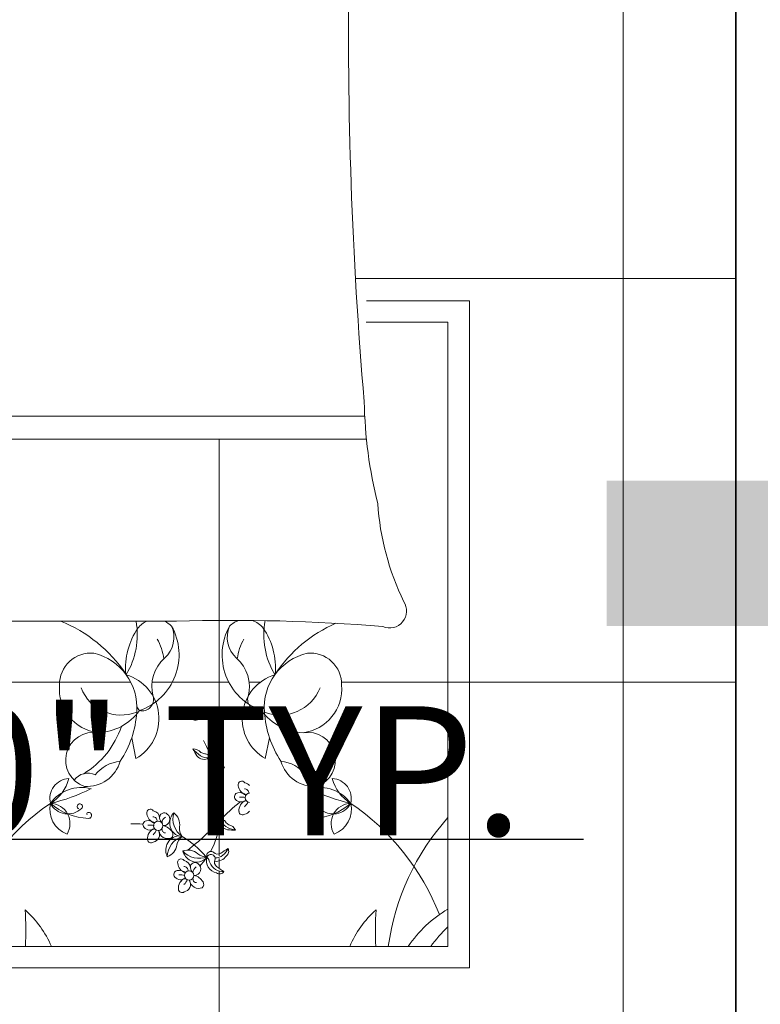
# Model space of a CAD drawing. Units: inches. Extents: x 351 to 1738, y -265 to 286.
# Tile 24 of 38: x 1200 to 1246, y 41 to 102. Entities that reach past the tile are written whole.
import ezdxf

# ---------------------------------------------------------------- set-up
doc = ezdxf.new("R2010")
doc.units = ezdxf.units.IN
doc.header["$MEASUREMENT"] = 0
for name, color, linetype, lineweight in [('A-ANNO-DIMS', 2, 'Continuous', 18), ('A-COLS-PATT', 6, 'Continuous', 13), ('A-FLOR-PATT', 9, 'Continuous', 9), ('A-FURN', 18, 'Continuous', 13), ('A-WALL', 7, 'Continuous', 35)]:
    doc.layers.add(name, color=color, linetype=linetype, lineweight=lineweight)
doc.styles.get("Standard").update_dxf_attribs({"font": 'arial.ttf'})
doc.dimstyles.get("Standard").update_dxf_attribs({"dimtxt": 8, "dimasz": 5, "dimexe": 0.18, "dimexo": 0.0625, "dimgap": 0.09, "dimtad": 1, "dimtoh": 1, "dimzin": 0, "dimdsep": 46, "dimlunit": 4, "dimtxsty": 'Standard', "dimcen": 0, "dimclre": 256, "dimadec": 0, "dimazin": 0, "dimtfac": 1, "dimtofl": 0, "dimtmove": 0, "dimatfit": 3, "dimfxl": 1, "dimtolj": 1, "dimtzin": 0, "dimlwe": -1, "dimarcsym": 0})

# ---------------------------------------------------------------- blocks, each defined once
blk = doc.blocks.new('*D52')
at = {"layer": 'A-ANNO-DIMS', "color": 0, "lineweight": -2, "transparency": 16777216}
for p, q in [((1098.304, 46.258), (1098.304, 51.258)), ((1098.304, 51.258), (1235.278, 51.258)), ((1098.304, 15.258), (1098.304, 41.258))]:
    blk.add_line(p, q, dxfattribs=at)
at = {"layer": 'A-ANNO-DIMS', "transparency": 16777216}
for p, q in [((1103.642, 46.258), (1098.124, 46.258)), ((1103.642, 10.258), (1098.124, 10.258))]:
    blk.add_line(p, q, dxfattribs=at)
at = {"layer": 'A-ANNO-DIMS', "color": 0, "transparency": 16777216}
for points in [[(1097.471, 41.258), (1099.137, 41.258), (1098.304, 46.258)], [(1097.471, 15.258), (1099.137, 15.258), (1098.304, 10.258)]]:
    blk.add_solid(points, dxfattribs=at)
at = {"layer": 'Defpoints', "color": 0, "transparency": 16777216}
for p in [(1098.304, 46.258), (1103.704, 46.258), (1103.704, 10.258)]:
    blk.add_point(p, dxfattribs=at)
at = {"layer": 'A-ANNO-DIMS', "color": 0, "transparency": 16777216, "insert": (1166.836, 55.49), "char_height": 8, "attachment_point": 5}
blk.add_mtext('\\A1;STAIR WINDOW 3\'-0" TYP.', dxfattribs=at)

msp = doc.modelspace()

# ---------------------------------------------------------------- hatches: boundary and pattern name
at = {"layer": 'A-COLS-PATT'}
h = msp.add_hatch(color=256, dxfattribs=at)
h.dxf.hatch_style = 1
h.paths.add_polyline_path([(1112.704, 237.963), (1103.704, 237.963), (1103.704, 228.963), (1112.704, 228.963)])
h.paths.add_polyline_path([(1115.704, 237.963), (1112.704, 237.963), (1112.704, 228.963), (1115.704, 228.963)])
h.paths.add_polyline_path([(1043.704, 255.963), (1034.704, 255.963), (1034.704, 243.963), (1043.704, 243.963)])
h.paths.add_polyline_path([(1043.704, 210.963), (1034.704, 210.963), (1034.704, 198.963), (1043.704, 198.963)])
h.paths.add_polyline_path([(1043.704, -45.037), (1034.704, -45.037), (1034.704, -57.037), (1043.704, -57.037)])
h.paths.add_polyline_path([(1112.704, -45.037), (1103.704, -45.037), (1103.704, -57.037), (1112.704, -57.037)])
h.paths.add_polyline_path([(1112.704, -161.037), (1103.704, -161.037), (1103.704, -164.037), (1103.704, -173.037), (1112.704, -173.037)])
h.paths.add_polyline_path([(1043.704, -161.037), (1034.704, -161.037), (1034.704, -173.037), (1043.704, -173.037)])
h.paths.add_polyline_path([(1248.549, -164.037), (1236.549, -164.037), (1236.549, -173.037), (1248.549, -173.037)])
h.paths.add_polyline_path([(1248.549, -50), (1236.549, -50), (1236.549, -59), (1248.549, -59)])
h.paths.add_polyline_path([(1248.704, 73.463), (1244.704, 73.463), (1244.704, 64.463), (1248.704, 64.463)])
h.paths.add_polyline_path([(1244.704, 73.463), (1236.704, 73.463), (1236.704, 64.463), (1244.704, 64.463)])
h.paths.add_polyline_path([(1248.704, 237.963), (1236.704, 237.963), (1236.704, 228.963), (1248.704, 228.963)])
h.paths.add_polyline_path([(1392.204, 237.963), (1380.204, 237.963), (1380.204, 228.963), (1392.204, 228.963)])
h.paths.add_polyline_path([(1536.064, 237.963), (1524.064, 237.963), (1524.064, 228.963), (1536.064, 228.963)])
h.paths.add_polyline_path([(1536.064, 73.463), (1524.064, 73.463), (1524.064, 64.463), (1536.064, 64.463)])
h.paths.add_polyline_path([(1384.204, 73.463), (1380.204, 73.463), (1380.204, 64.463), (1384.204, 64.463)])
h.paths.add_polyline_path([(1392.064, 73.463), (1384.204, 73.463), (1384.204, 64.463), (1392.064, 64.463)])
h.paths.add_polyline_path([(1536.064, -53.037), (1524.064, -53.037), (1524.064, -57.037), (1536.064, -57.037)])
h.paths.add_polyline_path([(1536.064, -48.037), (1524.064, -48.037), (1524.064, -53.037), (1536.064, -53.037)])
h.paths.add_polyline_path([(1392.064, -48.037), (1380.064, -48.037), (1380.064, -56.5), (1380.065, -57.037), (1392.064, -57.037)])
h.paths.add_polyline_path([(1536.064, -164.037), (1524.064, -164.037), (1524.064, -173.037), (1536.064, -173.037)])
at = {"layer": 'A-FLOR-PATT', "transparency": 33554559}
h = msp.add_hatch(dxfattribs=at)
h.set_pattern_fill('ANSI37', color=256, scale=200, angle=135)
h.set_pattern_definition([(180, (1112.704, -164.037), (-2e-15, -25), []), (270, (1112.704, -164.037), (25, -5e-15), [])])
h.paths.add_polyline_path([(1380.064, 73.463), (1380.132, 148.463), (1338.064, 148.463), (1290.704, 148.463), (1290.704, 88.463), (1248.704, 88.463), (1248.704, -2.009), (1244.704, -2.009), (1244.704, 142.457), (1160.704, 142.457), (1160.704, 158.963), (1160.704, 170.137), (1160.704, 206.137), (1160.704, 228.963), (1112.704, 228.963), (1112.704, 209.963), (1112.704, 168.963), (1124.704, 168.963), (1124.704, 162.963), (1112.704, 162.963), (1112.704, 64.463), (1112.704, 60.463), (1112.704, 0.463), (1112.704, -48.026), (1146.804, -47.981), (1146.804, -35.691), (1207.804, -35.691), (1207.804, -47.902), (1236.542, -47.864), (1236.544, -50.009), (1248.5, -50.009), (1248.506, -102.915), (1248.512, -150.915), (1248.514, -164.037), (1248.549, -164.037), (1273.017, -164.037), (1273.017, -128.799), (1355.24, -128.799), (1355.24, -164.037), (1384.204, -164.037), (1384.204, -57.037), (1380.064, -57.037), (1380.064, -48.037), (1392.064, -48.037), (1392.064, -53.037), (1406.549, -53.037), (1406.549, -57.037), (1401.204, -57.037), (1401.204, -147.037), (1468.204, -147.037), (1468.204, -138.5), (1472.204, -138.5), (1472.204, -102.5), (1468.204, -102.5), (1468.204, -57.037), (1442.549, -57.037), (1442.549, -53.037), (1463.049, -53.037), (1463.049, -40.747), (1524.049, -40.747), (1524.049, -48.037), (1536.064, -48.037), (1536.064, -53.037), (1557.704, -53.037), (1557.704, 204.963), (1384.204, 204.963), (1384.204, 73.463), (1392.064, 73.463), (1392.064, 64.463), (1384.204, 64.463), (1384.204, -3.5), (1380.204, -3.537), (1380.204, 64.463), (1380.064, 64.463)])
h.paths.add_polyline_path([(1510.714, 86.458, -0.103984), (1511.661, 85.595, 0.470438), (1510.158, 87.614, 0.0961)], flags=16)
h.paths.add_polyline_path([(1510.443, 100.266, 0.009798), (1504.693, 100.48, 0.02879), (1504.6, 99.767, -0.165331), (1505.519, 96.135, -0.143601)], flags=16)
h.paths.add_polyline_path([(1487.201, 85.595, -0.103984), (1488.148, 86.458, 0.0961), (1488.704, 87.614, 0.470438)], flags=0)
h.paths.add_polyline_path([(1495.052, 100.43), (1494.178, 100.43, -0.026463), (1494.262, 99.774, -0.144219)], flags=16)
h.paths.add_polyline_path([(1444.485, 86.458, -0.103984), (1445.433, 85.595, 0.470438), (1443.93, 87.614, 0.0961)], flags=16)
h.paths.add_polyline_path([(1420.972, 85.595, -0.103984), (1421.92, 86.458, 0.0961), (1422.475, 87.614, 0.470438)], flags=16)
h.paths.add_polyline_path([(1428.632, 100.335, 0.001054), (1427.971, 100.309, -0.021524), (1428.033, 99.774, -0.114301)], flags=16)
h.paths.add_polyline_path([(1419.906, 143.708, 0.024979), (1420.222, 157.526), (1421.573, 159.101), (1421.573, 175.369), (1391.393, 175.369), (1391.393, 200.519), (1542.294, 200.519), (1542.294, 175.369), (1512.028, 175.369, 0.019865), (1511.521, 153.838, 0.025134), (1512.758, 118.323, 0.020553), (1512.942, 115.253), (1419.834, 115.253, -0.000414), (1419.843, 124.798), (1413.059, 124.798), (1413.059, 84.437, -0.061853), (1415.831, 80.45, -0.093077), (1420.972, 85.595, -0.267537), (1422.371, 84.732, 0.08511), (1424.052, 84.616, -0.885393), (1424.033, 84.851, -1.125815), (1424.073, 84.366, -0.087987), (1422.371, 84.732, -0.267537), (1422.326, 83.089, -0.370542), (1420.972, 85.595, 0.093077), (1415.831, 80.45, -0.087414), (1417.914, 73.937), (1418.941, 73.937, 0.02725), (1418.913, 76.906, -0.115703), (1421.051, 73.937), (1445.354, 73.937, -0.115703), (1447.492, 76.906, 0.02725), (1447.464, 73.937), (1448.491, 73.937, -0.087414), (1450.574, 80.45, 0.093077), (1445.433, 85.595, -0.370542), (1444.079, 83.089, -0.267537), (1444.034, 84.732, -0.087987), (1442.332, 84.366, -1.125815), (1442.372, 84.851, -2.032736), (1442.364, 84.368, 0.086378), (1444.034, 84.732, -0.267537), (1445.433, 85.595, -0.093077), (1450.574, 80.45, -0.257732), (1466.483, 90.927, -0.47867), (1468.832, 91.907, -0.47867), (1471.18, 90.927, -0.26264), (1483.053, 81.78, -0.071866), (1487.201, 85.595, -0.267537), (1488.6, 84.732, 0.08511), (1490.28, 84.616, -0.885393), (1490.262, 84.851, -1.125815), (1490.301, 84.366, -0.087987), (1488.6, 84.732, -0.267537), (1488.554, 83.089, -0.370542), (1487.201, 85.595, 0.071866), (1483.053, 81.78, -0.132065), (1484.143, 73.937), (1485.169, 73.937, 0.02725), (1485.142, 76.906, -0.115703), (1487.28, 73.937), (1511.582, 73.937, -0.115703), (1513.72, 76.906, 0.02725), (1513.693, 73.937), (1514.719, 73.937, -0.087414), (1516.802, 80.45, 0.093077), (1511.661, 85.595, -0.370542), (1510.308, 83.089, -0.267537), (1510.262, 84.732, -0.087987), (1508.561, 84.366, -1.125815), (1508.601, 84.851, -2.032736), (1508.592, 84.368, 0.086378), (1510.262, 84.732, -0.267537), (1511.661, 85.595, -0.093077), (1516.802, 80.45, -0.061853), (1519.575, 84.437), (1519.575, 73.937), (1413.059, 73.937), (1413.059, 124.798), (1419.843, 124.798, -0.000821)], flags=16)
h.paths.add_polyline_path([(1220.149, 54.133, -0.103984), (1220.869, 53.476, 0.470438), (1219.727, 55.011, 0.0961)], flags=16)
h.paths.add_polyline_path([(1219.944, 64.626, 0.009798), (1215.574, 64.789, 0.02879), (1215.503, 64.247, -0.165331), (1216.201, 61.487, -0.143601)], flags=16)
h.paths.add_polyline_path([(1209.779, 64.449, 0.097446), (1209.339, 64.751), (1208.247, 64.751, 0.12739), (1207.7, 64.326, 0.171586), (1206.95, 61.475, -0.158854), (1207.636, 59.45, 0.015898), (1207.795, 59.218, 0.061546), (1208.598, 59.616, 0.175416), (1208.638, 60.099, -0.284779), (1209.348, 62.472, 0.326216)], flags=16)
h.paths.add_polyline_path([(1169.818, 54.133, -0.103984), (1170.538, 53.476, 0.470438), (1169.396, 55.011, 0.0961)], flags=16)
h.paths.add_polyline_path([(1159.017, 62.472, 0.284764), (1158.307, 60.099, -0.175433), (1158.267, 59.616, 0.39293), (1159.448, 64.449, -0.32623)], flags=16)
h.paths.add_polyline_path([(1156.342, 58.239, -0.178321), (1154.011, 55.31, -0.174736), (1154.722, 55.233, -0.200802), (1156.27, 56.086, 0.12699), (1157.283, 58.991, -0.091205)], flags=16)
h.paths.add_polyline_path([(1156.624, 61.413, 0.157275), (1157.316, 64.247, 0.169622)], flags=16)
h.paths.add_polyline_path([(1152.67, 54.133, -0.0961), (1151.95, 53.476, 0.064076), (1154.465, 54.384, 0.199016)], flags=16)
h.paths.add_polyline_path([(1202.281, 53.476, -0.103984), (1203, 54.133, 0.0961), (1203.423, 55.011, 0.470438)], flags=0)
h.paths.add_polyline_path([(1151.139, 97.64, 0.024979), (1151.379, 108.141), (1152.406, 109.338), (1152.406, 121.701), (1129.47, 121.701), (1129.47, 140.814), (1244.149, 140.814), (1244.149, 121.701), (1221.148, 121.701, 0.019865), (1220.763, 105.338, 0.025134), (1221.703, 78.349, 0.020553), (1221.843, 76.016), (1151.078, 76.016, -0.128743), (1148.786, 65.037, 0.539352), (1150.327, 64.171, -0.027594), (1163.481, 64.751, 0.097695), (1163.04, 64.449, 0.326216), (1163.471, 62.472, -0.284777), (1164.181, 60.099, -0.194757), (1165.846, 61.443, -0.155402), (1165.172, 64.247, -0.166022), (1165.869, 61.475, -0.177014), (1167.852, 62.77, -0.448203), (1169.974, 60.807, -0.393499), (1167.679, 57.86, -0.895548), (1168.438, 54.524, -0.355767), (1166.218, 56.086, -0.066024), (1165.505, 57.539), (1165.251, 56.243, -0.371732), (1164.02, 59.758, -0.373614), (1163.04, 64.449, -0.097695), (1163.481, 64.751, 0.021354), (1153.294, 64.429, -0.134183), (1156.695, 61.368, 0.186873), (1154.636, 62.77, 0.448203), (1152.514, 60.807, 0.403726), (1154.905, 57.846, 0.711219), (1153.334, 55, 0.53154), (1151.95, 53.476, -0.267537), (1153.013, 52.821, 0.08511), (1154.29, 52.732, -0.885393), (1154.276, 52.911, -1.125815), (1154.306, 52.543, -0.087987), (1153.013, 52.821, -0.267537), (1152.978, 51.572, -0.370542), (1151.95, 53.476, 0.093077), (1148.043, 49.566, -0.087414), (1149.626, 44.617), (1150.406, 44.617, 0.02725), (1150.385, 46.873, -0.115703), (1152.01, 44.617), (1170.478, 44.617, -0.115703), (1172.103, 46.873, 0.02725), (1172.082, 44.617), (1172.862, 44.617, -0.087414), (1174.445, 49.566, 0.093077), (1170.538, 53.476, -0.370542), (1169.51, 51.572, -0.267537), (1169.475, 52.821, -0.087987), (1168.182, 52.543, -1.125815), (1168.212, 52.911, -2.032736), (1168.206, 52.544, 0.086378), (1169.475, 52.821, -0.267537), (1170.538, 53.476, -0.093077), (1174.445, 49.566, -0.257732), (1186.536, 57.528, -0.47867), (1188.321, 58.273, -0.47867), (1190.106, 57.528, -0.26264), (1199.128, 50.577, -0.071866), (1202.281, 53.476, -0.267537), (1203.344, 52.821, 0.08511), (1204.621, 52.732, -0.885393), (1204.607, 52.911, -1.125815), (1204.637, 52.543, -0.087987), (1203.344, 52.821, -0.267537), (1203.309, 51.572, -0.370542), (1202.281, 53.476, 0.071866), (1199.128, 50.577, -0.132065), (1199.957, 44.617), (1200.737, 44.617, 0.02725), (1200.716, 46.873, -0.115703), (1202.341, 44.617), (1220.809, 44.617, -0.115703), (1222.434, 46.873, 0.02725), (1222.413, 44.617), (1223.193, 44.617, -0.087414), (1224.776, 49.566, 0.093077), (1220.869, 53.476, -0.370542), (1219.841, 51.572, -0.267537), (1219.806, 52.821, -0.087987), (1218.513, 52.543, -1.125815), (1218.543, 52.911, -2.032736), (1218.537, 52.544, 0.086378), (1219.806, 52.821, -0.267537), (1220.869, 53.476, -0.093077), (1224.776, 49.566, -0.061853), (1226.883, 52.597), (1226.883, 44.617), (1145.936, 44.617), (1145.936, 83.269), (1151.091, 83.269, -0.000821)], flags=16)
h.paths.add_polyline_path([(1218.01, 57.86, -0.895548), (1218.769, 54.524, -0.355767), (1216.549, 56.086, -0.066024), (1215.836, 57.539), (1215.582, 56.243, -0.371732), (1214.351, 59.758, -0.373614), (1213.371, 64.449, 0.326216), (1213.802, 62.472, -0.284777), (1214.512, 60.099, -0.194757), (1216.177, 61.443, -0.179991), (1218.183, 62.77, -0.448203), (1220.305, 60.807, -0.393499)], flags=16)
h.paths.add_polyline_path([(1424.735, 91.363, -0.393499), (1421.715, 95.241, -0.448203), (1424.507, 97.824, -0.179991), (1427.147, 96.077, -0.194757), (1429.338, 94.309, -0.284777), (1430.272, 97.432, 0.326216), (1430.839, 100.034, -0.373614), (1429.55, 93.861, -0.371732), (1427.929, 89.235), (1427.596, 90.941, -0.066024), (1426.657, 89.029, -0.355767), (1423.736, 86.973, -0.895548)], flags=16)
h.paths.add_polyline_path([(1238.033, 131.257, -1), (1227.329, 131.257, -1)], flags=0)
h.paths.add_polyline_path([(1235.357, 131.257, -1), (1230.005, 131.257, -1)], flags=0)
h.paths.add_polyline_path([(1214.039, 54.243, 0.154382), (1214.38, 53.992, 0.358955), (1213.613, 54.016, 0.603948), (1214.379, 53.657, 0.371319), (1213.968, 52.872, 0.187994), (1214.312, 52.809, -0.592455), (1213.953, 52.967, -0.294279), (1214.083, 53.691, -1.300187), (1213.881, 54.134, -0.283762), (1214.469, 53.896, 1.15094)], flags=16)
h.paths.add_polyline_path([(1212.091, 56.286, -0.408434), (1211.337, 56.445, -0.036259), (1211.098, 56.848, -0.236098), (1211.59, 56.63, 0.035345), (1211.835, 56.543, -0.475241), (1212.091, 56.286, -0.475241), (1212.438, 56.182, 0.035345), (1212.631, 56.007, -0.236098), (1213.056, 55.676, -0.036259), (1212.588, 55.697, -0.408434)], flags=16)
h.paths.add_polyline_path([(1211.469, 50.297, 0.296043), (1210.47, 50.527, 0.310883), (1211.931, 50.148, 0.021255)], flags=16)
h.paths.add_polyline_path([(1213.739, 51.818, -0.036259), (1213.271, 51.838, -0.408434), (1212.774, 52.427, -0.094786), (1212.293, 50.703, 1.150474), (1212.911, 50.232, 0.166288), (1213.265, 50.68, -0.025254), (1212.603, 50.13, 1.087932), (1212.471, 49.407, 0.166288), (1213.02, 49.251, -0.016128), (1212.567, 49.563, -0.286859), (1212.217, 49.638, 0.022156), (1212.046, 50.055, -0.64613), (1212.185, 50.498, 0.088412), (1212.732, 52.077, -1.186037), (1213.121, 52.323, 0.035345), (1213.314, 52.148, -0.236098)], flags=16)
h.paths.add_polyline_path([(1212.094, 50.342, -0.048524), (1211.54, 49.605, -1.103834), (1211.397, 48.738, -0.785515), (1211.683, 48.254, -0.392043), (1210.948, 48.525, -0.392819), (1210.561, 47.995, -0.592455), (1210.201, 48.153, -0.294279), (1210.331, 48.877, -0.704172), (1210.316, 49.592, -0.679344), (1210.729, 50.112, 0.563676)], flags=16)
h.paths.add_polyline_path([(1211.274, 49.829, -0.139826), (1210.745, 49.859, -0.217879), (1210.948, 49.509, -0.498572)], flags=0)
h.paths.add_polyline_path([(1433.426, 81.49, -0.181571), (1434.245, 81.788, -0.008067), (1433.726, 82.205, 0.045578), (1432.755, 81.242, 0.179011)], flags=16)
h.paths.add_polyline_path([(1434.146, 81.009, -0.132442), (1433.645, 80.771, 0.259089), (1433.234, 80.471, -0.180211), (1433.392, 80.805, -0.16994), (1432.758, 81.109, 0.032652), (1433.273, 80.474, -0.493363), (1434.046, 80.146, -0.390497)], flags=16)
h.paths.add_polyline_path([(1434.83, 80.047, -0.947538), (1435.294, 79.576, -0.299128), (1434.625, 79.404, -0.270439), (1435.01, 78.591, -0.592455), (1434.537, 78.382, -0.392819), (1434.027, 79.08, -0.392043), (1433.06, 78.723, -0.352042), (1433.003, 79.197, -0.197216), (1433.75, 79.734, -0.71364), (1434.447, 79.939, -0.21479), (1434.819, 80.475, 0.408833), (1435.075, 80.803, -0.226152)], flags=16)
h.paths.add_polyline_path([(1432.67, 81.217, -0.454218), (1431.897, 79.923, -0.414411), (1431.301, 80.035, 0.016129), (1431.897, 80.445, 0.27957), (1432.073, 80.871, -0.289504), (1431.103, 81.321, -0.414411), (1430.978, 81.915, 0.01613), (1431.586, 81.521, 0.341293), (1432.125, 81.583, -0.813186)], flags=16)
h.paths.add_polyline_path([(1429.893, 86.381, -0.947538), (1430.358, 85.91, -0.173106), (1429.984, 85.712, -0.038817), (1431.625, 84.214, -0.0879), (1432.097, 88.549, -0.049768), (1431.254, 88.49, -0.236098), (1431.814, 88.925, 0.035345), (1432.067, 89.155, -0.475241), (1432.524, 89.291, -0.475241), (1432.86, 89.63, 0.035345), (1433.182, 89.744, -0.236098), (1433.83, 90.032, -0.036259), (1433.516, 89.502, -0.408434), (1432.524, 89.291, -0.312424), (1432.106, 88.58, 0.088559), (1431.625, 84.214, -0.408434), (1430.971, 83.439, -0.036259), (1430.355, 83.412, -0.236098), (1430.914, 83.847, 0.035345), (1431.168, 84.078, -0.475241), (1431.625, 84.214, 0.038817), (1429.984, 85.712, -0.321732), (1429.333, 86.048, -0.32743), (1429.883, 86.809, 0.408833), (1430.138, 87.138, -0.226152)], flags=16)
h.paths.add_polyline_path([(1211.206, 58.616, -0.999784), (1211.336, 59.323, -0.614994)], flags=16)
h.paths.add_polyline_path([(1210.288, 49.429, 0.154382), (1210.629, 49.178, 0.358955), (1209.861, 49.202, 0.603948), (1210.627, 48.843, -0.534825), (1210.806, 49.295, 0.748346)], flags=16)
h.paths.add_polyline_path([(1209.589, 51.828, -0.008791), (1209.775, 51.753, 0.112231), (1209.466, 52.019, 1.418851), (1209.014, 51.708, -0.458726), (1208.651, 51.073, -0.592455), (1208.291, 51.232, -0.294279), (1208.421, 51.955, -1.300187), (1208.219, 52.398, -0.226005), (1208.719, 52.257, -0.475519), (1209.158, 52.369, -1.455499), (1209.603, 52.664, 0.421305), (1209.191, 52.262, -0.591212), (1208.979, 51.796, 0.497399), (1209.773, 51.333, 0.649312)], flags=16)
h.paths.add_polyline_path([(1208.029, 52.041, 0.544667), (1208.832, 52.045, 0.220132)], flags=0)
h.paths.add_polyline_path([(1210.438, 51.425, -0.2042), (1210.277, 52.018, 0.270826), (1209.915, 52.897, 0.324115)], flags=0)
h.paths.add_polyline_path([(1209.668, 52.407, -0.60139), (1208.99, 52.221, -0.394916), (1208.248, 52.83, -0.836792), (1208.651, 53.017, -0.338488), (1209.039, 52.571, 0.194138), (1209.191, 52.262, 0.413995), (1209.712, 52.475, 0.51771), (1210.503, 51.416, 0.401922), (1209.493, 50.93, 0.206396), (1209.516, 50.165, -0.319463), (1210.417, 51.418, -0.466635)], flags=16)
h.paths.add_polyline_path([(1206.601, 56.086, -0.355767), (1204.381, 54.524, -0.921198), (1205.236, 57.846, 0.206569), (1207.614, 58.991, -0.12699)], flags=16)
h.paths.add_polyline_path([(1435.487, 82.816, 0.527765), (1436.615, 83.361, 0.50854), (1437.05, 82.433, 0.592455), (1437.524, 82.641, 0.331245), (1436.963, 83.548, 0.387863), (1437.808, 83.626, 0.592954), (1437.618, 84.176, 0.226016), (1436.961, 83.99, 0.318205), (1437.588, 84.854, 0.689374), (1437.05, 84.991, 0.335765), (1436.539, 84.41, -0.156993), (1436.404, 84.065, -0.434611), (1436.961, 83.99, -0.21479), (1437.333, 84.526, 0.408833), (1437.588, 84.854, -0.226152), (1437.343, 84.097, -0.947538), (1437.808, 83.626, -0.299128), (1437.139, 83.455, -0.270439), (1437.524, 82.641, -0.592455), (1437.05, 82.433, -0.392819), (1436.541, 83.13, -0.43966), (1435.475, 82.794, -0.174614), (1435.942, 82.244, -0.206396), (1435.912, 81.237, -0.270826), (1435.125, 82.208, 0.207976), (1434.686, 82.904, -0.196495)], flags=16)
h.paths.add_polyline_path([(1435.386, 84.832, 0.270811), (1434.91, 83.676, -0.204217), (1434.699, 82.895, 0.324115)], flags=0)
h.paths.add_polyline_path([(1435.68, 84.18, -0.217656), (1435.554, 83.304, -0.176705), (1436.236, 83.778, -0.373036)], flags=0)
h.paths.add_polyline_path([(1435.566, 100.034, 0.326216), (1436.133, 97.432, -0.284777), (1437.067, 94.309, -0.194757), (1439.258, 96.077, -0.155402), (1438.371, 99.767, -0.166022), (1439.289, 96.12, -0.177014), (1441.897, 97.824, -0.448203), (1444.69, 95.241, -0.393499), (1441.67, 91.363, -0.895548), (1442.669, 86.973, -0.355767), (1439.748, 89.029, -0.066024), (1438.809, 90.941), (1438.476, 89.235, -0.371732), (1436.855, 93.861, -0.373614)], flags=16)
h.paths.add_polyline_path([(1191.252, 49.507, -0.274022), (1190.658, 48.409, 0.267537), (1191.311, 47.344, 0.370542)], flags=0)
h.paths.add_polyline_path([(1190.301, 49.717, 0.199016), (1188.619, 49.04, 0.064076), (1191.252, 49.507, -0.0961)], flags=0)
h.paths.add_polyline_path([(1189.518, 47.857, 1.125815), (1189.676, 47.523, 2.044605)], flags=0)
h.paths.add_polyline_path([(1464.974, 80.372, 0.274022), (1465.756, 78.927, -0.083013)], flags=0)
h.paths.add_polyline_path([(1464.974, 80.372, 0.370542), (1464.897, 77.525, 0.576324)], flags=0)
h.paths.add_polyline_path([(1464.974, 80.372, -0.470438), (1467.284, 81.372, -0.0961), (1466.226, 80.648, -0.199016), (1468.439, 79.757, -0.064076)], flags=0)
h.paths.add_polyline_path([(1189.511, 56.43, -0.259467), (1188.321, 56.391, -0.259467), (1187.13, 56.43, 0.08511), (1188.193, 55.716, -0.885393), (1188.27, 55.878, -1.196013), (1188.355, 55.442, 0.101459)], flags=0)
h.paths.add_polyline_path([(1188.321, 57.596, 0.078072), (1187.678, 57.24, 0.01555), (1188.321, 57.136, 0.01555), (1188.964, 57.24, 0.078072)], flags=0)
h.paths.add_polyline_path([(1190.164, 55.365, -0.576324), (1190.106, 57.528, -0.198294), (1188.321, 58.319, -0.198294), (1186.536, 57.528, -0.576324), (1186.477, 55.365, -0.370542), (1186.536, 57.528, 0.198294), (1188.321, 58.319, 0.198294), (1190.106, 57.528, -0.370542)], flags=0)
h.paths.add_polyline_path([(1188.372, 55.878, 1.125814), (1188.529, 55.544, 2.044605)], flags=0)
h.paths.add_polyline_path([(1186.341, 49.717, -0.0961), (1185.389, 49.507, 0.064076), (1188.022, 49.04, 0.199016)], flags=0)
h.paths.add_polyline_path([(1185.389, 49.507, -0.267537), (1185.984, 48.409, 0.08511), (1187.046, 47.695, -0.885393), (1187.123, 47.857, -1.125815), (1186.966, 47.523, -0.087987), (1185.984, 48.409, -0.267537), (1185.331, 47.344, -0.370542)], flags=0)
h.paths.add_polyline_path([(1399.441, 187.944, -1), (1413.525, 187.944, -1)], flags=0)
h.paths.add_polyline_path([(1402.962, 187.944, -1), (1410.004, 187.944, -1)], flags=0)
h.paths.add_polyline_path([(1357.663, -72.245), (1377.272, -72.245), (1377.272, -91.854), (1357.663, -91.854)], flags=16)
h.paths.add_polyline_path([(1467.256, 78.201, -1.125815), (1467.049, 77.761, -2.044605)], flags=0)
h.paths.add_polyline_path([(1468.822, 88.714, 0.941125), (1469.106, 88.316, 1.137152), (1468.765, 88.755, 0.890986), (1468.99, 88.245, 0.094828), (1470.398, 89.481, -0.267537), (1471.18, 90.927, -0.028123), (1469.678, 90.547, -0.028774), (1469.948, 90.311, -0.020327), (1468.832, 90.41, -0.020327), (1467.716, 90.311, -0.028774), (1467.986, 90.547, -0.028123), (1466.483, 90.927, -0.267537), (1467.265, 89.481, 0.08511), (1468.663, 88.542, -1.202316)], flags=0)
h.paths.add_polyline_path([(1178.25, 124.523, -0.119929), (1165.65, 124.145, -0.107349), (1159.133, 124.446, -0.102891), (1159.132, 130.465, -0.074897), (1158.993, 137.956, 0.002027), (1167.844, 137.479, -0.07553), (1180.337, 137.666, -0.075861), (1186.502, 137.688, -0.14099), (1186.272, 130.046, -0.095481), (1186.729, 124.748, -0.10603)], flags=0)
h.paths.add_polyline_path([(1469.225, 79.757, -0.199016), (1471.437, 80.648, -0.0961), (1470.379, 81.372, -0.470438), (1472.689, 80.372, -0.370542), (1472.766, 77.525, -0.267537), (1471.907, 78.927, -0.087986), (1470.615, 77.761, -1.125849), (1470.408, 78.201, -2.032736), (1470.642, 77.778, 0.086378), (1471.907, 78.927, -0.267537), (1472.689, 80.372, -0.064076)], flags=0)
h.paths.add_polyline_path([(1430.423, 186.902, -0.074897), (1430.24, 196.758, 0.002027), (1441.887, 196.131, -0.07553), (1458.326, 196.377, -0.075861), (1466.438, 196.406, -0.14099), (1466.136, 186.35, -0.095481), (1466.737, 179.378, -0.10603), (1455.58, 179.082, -0.119929), (1439, 178.585, -0.107349), (1430.425, 178.981, -0.102891)], flags=0)
h.paths.add_polyline_path([(1162.258, 49.939, 0.335765), (1161.87, 49.497, -0.156994), (1161.767, 49.235, -0.434611), (1162.19, 49.178, -0.21479), (1162.473, 49.585, 1.529195)], flags=16)
h.paths.add_polyline_path([(1161.683, 49.021, 0.581518), (1161.268, 49.583, 0.592761)], flags=16)
h.paths.add_polyline_path([(1162.602, 48.058, 0.371319), (1162.192, 48.843, 0.434533), (1162.88, 48.962, 0.185081), (1162.197, 48.926, 1.121837)], flags=16)
h.paths.add_polyline_path([(1161.443, 48.941, -1.307104), (1161.495, 48.571, -0.217752), (1161.136, 48.254, 0.697303), (1161.871, 49.048, 0.121514)], flags=16)
h.paths.add_polyline_path([(1162.531, 49.429, -0.207084), (1162.05, 49.146, -0.99203)], flags=16)
h.paths.add_polyline_path([(1161.304, 49.578, -0.719667), (1161.513, 50.079, -0.130428), (1160.836, 50.168, 0.039593)], flags=0)
h.paths.add_polyline_path([(1162.036, 50.584, -0.008067), (1161.642, 50.9, 0.029367), (1161.35, 50.297, -0.205788)], flags=16)
h.paths.add_polyline_path([(1162.882, 51.392, -0.124733), (1162.763, 51.828, -0.101191), (1162.399, 51.438, -0.153425)], flags=0)
h.paths.add_polyline_path([(1164.235, 51.85, -0.309107), (1164.513, 51.136, -0.627125), (1163.781, 51.603, -0.685909), (1162.777, 51.219, -0.233285), (1163.303, 50.165, -0.270826), (1162.705, 50.903, 0.2042), (1162.381, 51.425, 0.204182), (1162.542, 52.018, -0.270841), (1162.903, 52.897, -0.127261), (1163.219, 52.529, -1.168681), (1163.781, 52.587, -0.329112), (1164.168, 53.017, -0.836792), (1164.571, 52.83, -0.193341), (1164.391, 52.338, -0.947538), (1164.744, 51.981, -0.299128)], flags=16)
h.paths.add_polyline_path([(1163.598, 51.937, -1.262956), (1163.236, 51.831, 0.012575), (1162.971, 51.721, 0.230657), (1163.151, 52.407, -0.164898), (1163.178, 52.661, -0.44932), (1163.628, 52.262, -0.721477), (1164.154, 52.088, -0.849998)], flags=0)
h.paths.add_polyline_path([(1161.613, 58.616, -0.980413), (1161.525, 59.049, -2.908935)], flags=16)
h.paths.add_polyline_path([(1160.252, 49.166, -0.414411), (1159.799, 49.251, 0.016129), (1160.252, 49.563, 0.27957), (1160.386, 49.887, -0.289504), (1159.649, 50.229, -0.414411), (1159.554, 50.68, 0.01613), (1160.015, 50.381, 0.617885), (1160.526, 50.703, -0.094786), (1160.045, 52.427, -0.140444), (1159.682, 52.042, -0.057856), (1159.3, 51.872, 0.544843), (1160.046, 52.419, -0.088122), (1160.404, 55.721, -0.049768), (1159.763, 55.676, -0.236098), (1160.188, 56.007, 0.035345), (1160.381, 56.182, -0.475241), (1160.728, 56.286, -0.475241), (1160.984, 56.543, 0.035345), (1161.229, 56.63, -0.236098), (1161.721, 56.848, -0.036259), (1161.482, 56.445, -0.408434), (1160.728, 56.286, -0.312424), (1160.411, 55.745, 0.088559), (1160.045, 52.427, 0.107081), (1160.634, 50.498, -0.494798), (1160.839, 50.149, -0.454218)], flags=16)
h.paths.add_polyline_path([(1160.666, 49.808, -2.076528), (1160.828, 50.172, 0.019586)], flags=0)
h.paths.add_polyline_path([(1158.439, 53.992, 0.154382), (1158.78, 54.243, 0.748346), (1158.262, 54.109, -0.338225), (1158.492, 53.839, -0.170816), (1159.124, 53.779, 0.495729), (1158.938, 54.134, 0.226016)], flags=16)
h.paths.add_polyline_path([(1160.045, 52.427, 0.038817), (1158.798, 53.565, -0.119818), (1158.574, 53.586, -0.309107), (1158.851, 52.872, -0.187994), (1158.506, 52.809, 0.592455), (1158.866, 52.967, 0.331245), (1158.44, 53.657, 0.201245), (1158.798, 53.565, -0.034023), (1159.901, 52.578, -0.044253), (1159.698, 52.323, -0.475241)], flags=16)
h.paths.add_polyline_path([(1336.926, -95.392), (1336.926, -117.945), (1291.82, -117.945), (1291.82, -95.392)], flags=16)
h.paths.add_polyline_path([(1357.535, -97.244), (1357.726, -96.697, 0.034844)], flags=16)
h.paths.add_polyline_path([(1376.693, -96.478), (1377.301, -96.5, 0.031497), (1375.907, -96.424), (1357.726, -96.424)], flags=16)
h.paths.add_polyline_path([(1379.403, -119.667, 0.026706), (1380.043, -119.439, -0.015299)], flags=16)
h.paths.add_polyline_path([(1357.726, -120.202), (1357.821, -120.202), (1357.821, -120.201)], flags=16)
h.paths.add_polyline_path([(1354.171, -104.592), (1354.469, -98.672, 0.011138)], flags=16)
h.paths.add_polyline_path([(1355.058, -119.136), (1354.578, -118.539, 0.143164)], flags=16)
h.paths.add_polyline_path([(1378.851, -96.821), (1378.85, -96.82), (1378.85, -96.82, -0.04968), (1380.055, -97.191), (1378.85, -96.82, 0.150054), (1375.135, -97.188), (1375.136, -119.44, -0.00997), (1374.747, -116.649), (1357.726, -116.649, 0.169385), (1357.535, -119.382), (1357.535, -119.382), (1357.535, -119.382, 0.034818), (1357.726, -119.928), (1357.726, -119.928), (1357.726, -119.929, -0.034877), (1357.535, -119.382), (1355.507, -119.382), (1355.317, -119.278), (1357.535, -119.382, -0.169394), (1357.726, -116.649, -0.039151), (1374.686, -116.113, -0.002015), (1374.625, -115.546, 0.115322), (1369.915, -115.474, 0.060921), (1369.922, -101.154, 0.115146), (1374.625, -101.079, -0.002016), (1374.686, -100.513, -0.039151), (1357.726, -99.977), (1374.747, -99.977, -0.009963), (1375.135, -97.188), (1375.135, -97.188, -0.150108)], flags=16)
h.paths.add_polyline_path([(1490.963, 91.363, -0.393499), (1487.944, 95.241, -0.448203), (1490.736, 97.824, -0.179991), (1493.376, 96.077, -0.194757), (1495.567, 94.309, -0.284777), (1496.501, 97.432, 0.326216), (1497.068, 100.034, -0.373614), (1495.778, 93.861, -0.371732), (1494.158, 89.235), (1493.824, 90.941, -0.066024), (1492.886, 89.029, -0.355767), (1489.964, 86.973, -0.895548)], flags=16)
h.paths.add_polyline_path([(1354.86, -97.658), (1355.316, -97.348, 0.101911)], flags=16)
h.paths.add_polyline_path([(1497.063, 83.327, 0.176724), (1496.37, 83.785, -0.405139), (1496.016, 83.384, 0.497399), (1497.06, 82.774, 0.649312), (1496.818, 83.426, -0.008791)], flags=16)
h.paths.add_polyline_path([(1496.339, 83.783, 0.592761), (1496.886, 84.522, 0.581518)], flags=16)
h.paths.add_polyline_path([(1495.11, 82.641, 0.592455), (1495.583, 82.433, 0.676915), (1495.805, 83.59, 0.375669)], flags=16)
h.paths.add_polyline_path([(1495.015, 84.176, -0.145057), (1495.301, 84.526, -0.408833), (1495.045, 84.854, 0.220629), (1495.381, 84.152, -0.199594), (1495.851, 83.764, -0.524017), (1494.826, 83.626, -0.592998)], flags=16)
h.paths.add_polyline_path([(1501.655, 81.915, -0.016129), (1501.048, 81.521, -0.392719), (1500.462, 81.37, -0.21067), (1500.607, 81.142, 0.306699)], flags=16)
h.paths.add_polyline_path([(1500.11, 89.291, -0.408434), (1499.118, 89.502, -0.036259), (1498.803, 90.032, -0.236098), (1499.451, 89.744, 0.035345), (1499.774, 89.63, -0.475241), (1500.11, 89.291, -0.475241), (1500.567, 89.155, 0.035345), (1500.82, 88.925, -0.236098), (1501.379, 88.49, -0.036259), (1500.763, 88.516, -0.408434)], flags=16)
h.paths.add_polyline_path([(1498.908, 82.205, -0.051322), (1500.013, 81.134, -0.587931), (1500.234, 81.676, 0.107081), (1501.009, 84.214, -0.03529)], flags=16)
h.paths.add_polyline_path([(1496.93, 83.875, -0.206396), (1497.247, 84.832, -0.270826), (1497.724, 83.676, 0.207976), (1497.944, 82.884, -0.381455)], flags=16)
h.paths.add_polyline_path([(1496.721, 81.237, 0.270812), (1497.509, 82.208, -0.204216), (1497.935, 82.895, 0.324115)], flags=16)
h.paths.add_polyline_path([(1497.529, 80.125, -0.145057), (1497.814, 80.475, -0.703182), (1498.282, 81.178, -0.122925), (1497.977, 81.714, -0.270837), (1499.207, 81.49, 0.207964), (1499.993, 81.248, -0.265145), (1499.278, 80.472, 0.381901), (1498.808, 79.947, -0.305905), (1498.848, 79.519, 0.499482), (1498.574, 79.217, -0.458726), (1498.097, 78.382, -0.592455), (1497.624, 78.591, -0.270439), (1498.009, 79.404, -0.299116), (1497.34, 79.576, -0.593016)], flags=16)
h.paths.add_polyline_path([(1500.736, 79.923, 0.414411), (1501.333, 80.035, -0.321648), (1500.192, 80.765, 0.019886), (1499.976, 81.251, 0.465331)], flags=16)
h.paths.add_polyline_path([(1501.009, 84.214, -0.038817), (1502.649, 85.712, -0.173095), (1502.276, 85.91, -0.593016), (1502.465, 86.46, -0.145057), (1502.751, 86.809, -0.408833), (1502.495, 87.138, 0.220629), (1502.831, 86.436, -0.199594), (1503.301, 86.048, -0.321732), (1502.649, 85.712, 0.038817), (1501.009, 84.214, 0.122449), (1501.412, 83.755, 0.475491), (1501.335, 84.226, 0.055822), (1501.719, 83.847, -0.236098), (1502.278, 83.412, -0.036259), (1501.663, 83.439, -0.408434)], flags=16)
h.paths.add_polyline_path([(1501.794, 100.034, 0.326216), (1502.362, 97.432, -0.284777), (1503.295, 94.309, -0.194757), (1505.486, 96.077, -0.179991), (1508.126, 97.824, -0.448203), (1510.918, 95.241, -0.393499), (1507.899, 91.363, -0.895548), (1508.898, 86.973, -0.355767), (1505.976, 89.029, -0.066024), (1505.038, 90.941), (1504.704, 89.235, -0.371732), (1503.084, 93.861, -0.373614)], flags=16)
h.paths.add_polyline_path([(1146.29, 131.257, -1), (1135.587, 131.257, -1)], flags=0)
h.paths.add_polyline_path([(1143.614, 131.257, -1), (1138.262, 131.257, -1)], flags=0)
h.paths.add_polyline_path([(1524.064, 73.463), (1536.064, 73.463), (1536.064, 64.463), (1524.064, 64.463)], flags=16)
h.paths.add_polyline_path([(1520.162, 187.944, -1), (1534.246, 187.944, -1)], flags=0)
h.paths.add_polyline_path([(1530.725, 187.944), (1527.204, 187.944), (1527.204, 184.423, 0.414214)], flags=0)
h.paths.add_polyline_path([(1278.415, -91.154), (1331.067, -91.154), (1331.067, -80.583), (1278.415, -80.583)], flags=24)
h.paths.add_polyline_path([(1266.655, -79.354), (1354.738, -79.354), (1354.738, -67.817), (1266.655, -67.817)], flags=24)
h.paths.add_polyline_path([(1115.482, 206.184), (1155.098, 206.184), (1155.098, 217.714), (1115.482, 217.714)], flags=24)
h.paths.add_polyline_path([(1161.771, 8.501), (1222.466, 8.501), (1222.466, 19.079), (1161.771, 19.079)], flags=24)
h.paths.add_polyline_path([(1164.656, 18.795), (1210.615, 18.795), (1210.615, 30.324), (1164.656, 30.324)], flags=24)
h.paths.add_polyline_path([(1368.147, -32.882), (1379.362, -32.882), (1379.362, -21.733), (1368.147, -21.733)], flags=24)
h.paths.add_polyline_path([(1244.842, -31.012), (1256.057, -31.012), (1256.057, -19.863), (1244.842, -19.863)], flags=24)
h.paths.add_polyline_path([(1114.589, 195.739), (1156.517, 195.739), (1156.517, 206.31), (1114.589, 206.31)], flags=24)
h.paths.add_polyline_path([(1436.398, 37.632), (1505.131, 37.632), (1505.131, 48.203), (1436.398, 48.203)], flags=24)
h.paths.add_polyline_path([(1435.991, 47.919), (1507.906, 47.919), (1507.906, 59.456), (1435.991, 59.456)], flags=24)
h.paths.add_polyline_path([(1415.107, -124.896), (1457.038, -124.896), (1457.038, -114.318), (1415.107, -114.318)], flags=24)
h.paths.add_polyline_path([(1417.992, -114.602), (1457.609, -114.602), (1457.609, -103.073), (1417.992, -103.073)], flags=24)

# ---------------------------------------------------------------- linework, layer by layer
at = {"layer": 'A-FURN'}
for p, q in [((1221.734, 77.446), (1151.085, 77.446)), ((1221.843, 76.016), (1151.085, 76.016)), ((1210.09, 64.751), (1163.529, 64.751)), ((1207.568, 56.243), (1207.314, 57.539)), ((1215.582, 56.243), (1215.836, 57.539))]:
    msp.add_line(p, q, dxfattribs=at)
for points in [[(1221.852, 84.598), (1228.212, 84.598), (1228.212, 43.288), (1144.607, 43.288), (1144.607, 84.598), (1151.094, 84.598)], [(1151.091, 83.269), (1145.936, 83.269), (1145.936, 44.617), (1226.883, 44.617), (1226.883, 83.269), (1221.828, 83.269)]]:
    msp.add_lwpolyline(points, dxfattribs=at)
msp.add_lwpolyline([(1221.703, 78.349, 0.056112), (1222.535, 72.039, 0.095341), (1224.147, 65.962)], format="xyb", dxfattribs=at)
for centre in [(1208.957, 52.088), (1210.867, 49.009)]:
    msp.add_circle(centre, 0.292, dxfattribs=at)
for centre, radius, start, end in [((1489.524, 101.184), 268.793, 179.11454, 184.87351), ((1223.278, 65.38), 1.045, 246.52186, 33.82642), ((1199.725, 56.675), 8.679, 33.66712, 68.50587), ((1202.908, 63.902), 4.751, 328.82178, 10.28665), ((1208.793, 63.482), 1.381, 113.28564, 142.32497), ((1208.793, 63.482), 1.381, 44.45169, 66.71436), ((1213.602, -46.785), 111.591, 85.24024, 91.80351), ((1214.357, 63.482), 1.381, 106.63434, 135.54831), ((1214.357, 63.482), 1.381, 37.67503, 72.58143), ((1220.242, 63.902), 4.751, 169.24899, 211.17822), ((1223.425, 56.675), 8.679, 113.64533, 146.33288), ((1211.357, 61.839), 4.423, 145.78505, 184.73037), ((1206.588, 62.668), 3.655, 289.28218, 29.1751), ((1208.209, 63.756), 1.716, 311.56531, 23.83541), ((1216.562, 62.668), 3.655, 150.8249, 250.71782), ((1214.941, 63.756), 1.716, 156.16459, 228.43469), ((1211.793, 61.839), 4.423, 355.26963, 34.21495), ((1206.036, 62.007), 3.296, 7.43599, 29.91487), ((1217.114, 62.007), 3.296, 150.08513, 172.56401), ((1204.781, 60.843), 1.936, 84.48557, 181.05378), ((1204.187, 59.41), 3.449, 355.29334, 76.921), ((1210.908, 60.713), 2.351, 131.56531, 195.14713), ((1212.242, 60.713), 2.351, 344.85287, 48.43469), ((1218.963, 59.41), 3.449, 103.079, 184.70666), ((1218.369, 60.843), 1.936, 358.94622, 95.51443), ((1206.146, 58.714), 2.851, 299.90854, 73.1337), ((1217.004, 58.714), 2.851, 106.8663, 240.09146), ((1205.575, 60.566), 2.74, 174.94485, 262.88575), ((1206.652, 61.605), 2.661, 201.58187, 291.42215), ((1216.498, 61.605), 2.661, 248.57785, 338.41813), ((1217.575, 60.566), 2.74, 277.11425, 5.05515), ((1207.951, 59.913), 0.712, 257.30406, 15.14713), ((1215.199, 59.913), 0.712, 164.85287, 282.69594), ((1205.099, 61.175), 3.331, 272.3591, 324.04014), ((1211.357, 61.839), 4.423, 212.70113, 216.34448), ((1211.271, 58.969), 0.359, 79.58644, 259.56155), ((1211.793, 61.839), 4.423, 323.65552, 327.29887), ((1218.051, 61.175), 3.331, 215.95986, 267.6409), ((1201.482, 59.502), 6.154, 326.28828, 356.5076), ((1211.246, 58.833), 0.221, 259.56155, 77.29493), ((1221.668, 59.502), 6.154, 183.4924, 213.71172), ((1201.532, 59.938), 5.414, 301.26137, 341.7045), ((1221.618, 59.938), 5.414, 198.2955, 238.73863), ((1204.945, 56.15), 1.721, 80.26398, 250.86884), ((1203.297, 53.061), 9.498, 20.10592, 26.9968), ((1218.205, 56.15), 1.721, 289.13116, 99.73602), ((1211.126, 56.247), 0.602, 39.50559, 92.64212), ((1212.518, 57.975), 1.813, 218.43876, 238.83597), ((1213.992, 58.292), 3.234, 206.50636, 215.31021), ((1211.795, 56.75), 0.55, 216.52319, 302.46683), ((1212.077, 57.247), 0.961, 238.83597, 270.81412), ((1212.328, 58.318), 1.842, 246.39009, 254.48709), ((1211.858, 56.31), 0.234, 353.94573, 95.62162), ((1212.64, 56.244), 0.55, 175.71315, 261.65678), ((1212.222, 56.092), 0.234, 22.55835, 124.23425), ((1212.944, 56.727), 0.961, 207.36586, 239.34401), ((1213.77, 57.455), 1.842, 223.69288, 231.78988), ((1204.532, 56.668), 2.149, 265.96902, 344.3045), ((1206.847, 53.811), 2.289, 96.1662, 141.58255), ((1203.297, 53.061), 9.498, 356.17232, 16.41582), ((1213.378, 57.46), 1.813, 239.34401, 259.74122), ((1212.961, 58.909), 3.234, 262.86976, 271.67361), ((1212.512, 55.417), 0.602, 25.53786, 78.67439), ((1218.618, 56.668), 2.149, 195.6955, 274.03098), ((1216.303, 53.811), 2.289, 38.41745, 83.8338), ((1203.487, 53.771), 1.241, 92.95159, 193.72796), ((1200.949, 55.66), 2.558, 301.38267, 345.29688), ((1204.59, 54.285), 1.055, 63.97555, 143.26805), ((1218.56, 54.285), 1.055, 36.73195, 116.02445), ((1222.201, 55.66), 2.558, 194.70312, 238.61733), ((1219.663, 53.771), 1.241, 346.27204, 87.04841), ((1204.202, 52.092), 2.368, 75.46535, 144.23429), ((1200.01, 63.704), 10.476, 282.51726, 297.18239), ((1214.128, 54.623), 0.226, 35.0752, 194.76444), ((1214.606, 54.657), 0.702, 187.49685, 251.27373), ((1214.278, 54.1), 0.279, 358.13253, 88.89195), ((1214.215, 54.276), 0.487, 37.3642, 78.43627), ((1218.948, 52.092), 2.368, 35.76571, 104.53465), ((1223.14, 63.704), 10.476, 242.81761, 257.48274), ((1213.923, 53.886), 0.252, 99.6513, 222.32085), ((1214.09, 54.038), 0.478, 222.32085, 310.21108), ((1213.982, 53.538), 0.604, 46.34618, 99.6513), ((1214.629, 53.026), 0.679, 111.63824, 184.94696), ((1214.097, 52.911), 0.956, 74.28291, 96.91484), ((1214.619, 53.823), 0.292, 93.27684, 266.72316), ((1210.738, 41.118), 14.975, 124.38655, 158.59079), ((1203.903, 53.123), 1.661, 167.71153, 249.03868), ((1203.365, 54.045), 1.225, 207.6827, 313.77619), ((1204.773, 56.328), 3.787, 228.84017, 267.9352), ((1202.243, 52.226), 1.251, 328.46331, 88.28689), ((1204.101, 53.278), 0.162, 313.77619, 249.71835), ((1208.466, 52.888), 0.226, 35.0752, 194.76444), ((1220.717, 44.98), 10.888, 127.9541, 136.84587), ((1213.7, 53.925), 0.887, 312.38963, 336.57243), ((1218.377, 56.328), 3.787, 272.0648, 311.15983), ((1219.784, 54.045), 1.225, 226.22381, 332.3173), ((1219.067, 53.34), 0.0976, 290.26671, 226.22708), ((1220.907, 52.226), 1.251, 91.71311, 211.53669), ((1219.247, 53.123), 1.661, 290.96132, 12.28847), ((1212.412, 41.118), 14.975, 21.40921, 55.61345), ((1204.625, 52.822), 0.0903, 101.4834, 217.94089), ((1204.644, 52.729), 0.186, 267.9352, 101.4834), ((1208.944, 52.922), 0.702, 187.49685, 251.27373), ((1208.617, 52.364), 0.279, 358.13253, 88.89195), ((1208.553, 52.54), 0.487, 3.63497, 78.43627), ((1209.324, 52.602), 0.286, 48.29465, 186.24744), ((1209.497, 52.605), 0.459, 184.21229, 228.15875), ((1209.593, 52.262), 0.402, 118.84925, 179.93549), ((1209.279, 52.494), 0.398, 268.57189, 53.89544), ((1210.638, 52.254), 0.967, 138.34199, 184.98936), ((1211.193, 52.522), 1.331, 163.63009, 235.46314), ((1209.345, 52.148), 0.942, 352.07481, 52.68955), ((1212.905, 52.234), 0.234, 22.55835, 124.23425), ((1214.176, 52.987), 0.224, 184.94696, 307.52629), ((1214.221, 53.282), 0.482, 280.95974, 322.23791), ((1218.506, 52.729), 0.186, 78.5166, 272.0648), ((1218.525, 52.822), 0.0903, 322.05911, 78.5166), ((1238.032, 42.599), 14.975, 138.1144, 172.25504), ((1207.539, 46.497), 5.712, 85.24147, 92.89291), ((1208.261, 52.15), 0.252, 99.6513, 222.32085), ((1208.429, 52.302), 0.478, 222.32085, 310.21108), ((1208.32, 51.803), 0.604, 46.34618, 99.6513), ((1208.967, 51.29), 0.679, 111.63824, 184.94696), ((1208.435, 51.175), 0.956, 74.28291, 96.91484), ((1208.039, 52.189), 0.887, 312.38963, 336.57243), ((1209.39, 51.841), 0.193, 172.86802, 277.09399), ((1209.035, 51.205), 0.921, 31.9501, 75.24419), ((1210.482, 52.224), 0.809, 183.87739, 267.15012), ((1211.053, 51.91), 0.783, 172.07481, 218.23927), ((1201.174, 62.961), 15.669, 307.82556, 317.75876), ((1208.029, 52.822), 4.762, 330.79592, 355.24398), ((1213.323, 52.386), 0.55, 175.71315, 261.65678), ((1213.627, 52.869), 0.961, 207.36586, 239.34401), ((1214.453, 53.596), 1.842, 223.69288, 231.78988), ((1214.062, 53.601), 1.813, 239.34401, 259.74122), ((1213.644, 55.05), 3.234, 262.86976, 271.67361), ((1213.195, 51.558), 0.602, 25.53786, 78.67439), ((1208.514, 51.251), 0.224, 184.94696, 307.52629), ((1208.559, 51.547), 0.482, 280.95974, 28.78041), ((1209.552, 51.865), 0.576, 188.56141, 292.59143), ((1210.251, 50.646), 0.809, 91.4625, 159.4747), ((1210.847, 50.158), 1.331, 107.88895, 179.722), ((1209.571, 51.539), 0.289, 314.37319, 31.9501), ((1207.539, 46.497), 5.712, 66.15226, 66.94993), ((1210.889, 50.784), 0.783, 125.11283, 171.27729), ((1207.539, 46.497), 5.712, 40.18202, 59.45598), ((1210.392, 50.574), 0.967, 158.36273, 205.0101), ((1209.183, 51.046), 0.942, 290.66254, 351.27729), ((1212.433, 50.974), 0.883, 272.31716, 340.52013), ((1208.395, 57.685), 8.532, 301.11559, 304.8118), ((1212.992, 50.502), 0.326, 303.09787, 33.13641), ((1210.376, 49.809), 0.226, 35.0752, 194.76444), ((1210.792, 49.642), 0.942, 49.38119, 109.99593), ((1211.476, 51.399), 1.331, 220.93647, 292.76952), ((1211.401, 50.788), 0.967, 195.64837, 242.29574), ((1211.342, 50.64), 0.809, 241.18377, 321.67918), ((1211.915, 50.952), 0.783, 229.38119, 275.54564), ((1208.029, 52.822), 4.762, 317.50829, 325.99666), ((1212.703, 49.914), 0.76, 162.8042, 259.69432), ((1212.216, 50.245), 0.255, 45.73542, 228.12966), ((1212.217, 50.054), 0.255, 338.24522, 160.63946), ((1207.427, 47.925), 5.087, 21.70871, 26.21806), ((1212.629, 50.67), 0.338, 225.73542, 301.11559), ((1212.531, 50.641), 0.76, 262.60083, 327.18452), ((1210.854, 49.843), 0.702, 187.49685, 251.27373), ((1210.527, 49.286), 0.279, 358.13253, 88.89195), ((1210.463, 49.462), 0.487, 3.63497, 78.43627), ((1211.234, 49.524), 0.286, 48.29465, 186.24744), ((1211.408, 49.526), 0.459, 184.21229, 228.15875), ((1211.503, 49.184), 0.402, 118.84925, 179.93549), ((1211.19, 49.415), 0.398, 268.57189, 53.89544), ((1212.974, 50.133), 0.883, 201.70871, 273.02993), ((1212.767, 49.835), 0.338, 158.24522, 233.62539), ((1217.627, 56.433), 8.532, 233.62539, 237.3216), ((1210.172, 49.072), 0.252, 99.6513, 222.32085), ((1210.339, 49.224), 0.478, 222.32085, 310.21108), ((1210.231, 48.724), 0.604, 46.34618, 99.6513), ((1210.878, 48.212), 0.679, 111.63824, 184.94696), ((1210.345, 48.097), 0.956, 74.28291, 96.91484), ((1211.3, 48.763), 0.193, 172.86802, 277.09399), ((1210.945, 48.127), 0.921, 31.9501, 75.24419), ((1212.751, 49.435), 0.326, 235.60767, 325.6462), ((1209.949, 49.111), 0.887, 312.38963, 336.57243), ((1210.469, 48.468), 0.482, 280.95974, 28.78041), ((1211.462, 48.786), 0.576, 188.56141, 292.59143), ((1211.481, 48.461), 0.289, 314.37319, 31.9501), ((1210.425, 48.173), 0.224, 184.94696, 307.52629), ((1180.038, 45.554), 20.719, 357.40811, 3.65191), ((1196.717, 42.281), 6.089, 22.55474, 48.95456), ((1226.433, 42.281), 6.089, 131.04544, 157.44526), ((1243.112, 45.554), 20.719, 176.34809, 182.59189), ((1230.519, 40.593), 7.297, 119.88843, 146.53828), ((1233.145, 39.233), 9.094, 133.51858, 143.69643)]:
    msp.add_arc(centre, radius, start, end, dxfattribs=at)
at = {"layer": 'A-WALL'}
msp.add_line((1244.704, -2.009), (1244.704, 158.963), dxfattribs=at)

# ---------------------------------------------------------------- dimensions: what is measured, and where the dimension line sits
at = {"layer": 'A-ANNO-DIMS'}
dim = msp.add_linear_dim(base=(1098.304, 46.258), p1=(1103.704, 10.258), p2=(1103.704, 46.258), angle=90, text='STAIR WINDOW <> TYP.', dimstyle='Standard', override={"dimdec": 1, "dimlfac": 1, "dimrnd": 0, "dimzin": 1, "dimdsep": 46, "dimlunit": 4, "dimfrac": 2}, dxfattribs=at)
dim.commit()
dim.dimension.update_dxf_attribs({"geometry": '*D52', "text_midpoint": (1166.836, 55.49)})

doc.saveas('drawing.dxf')
